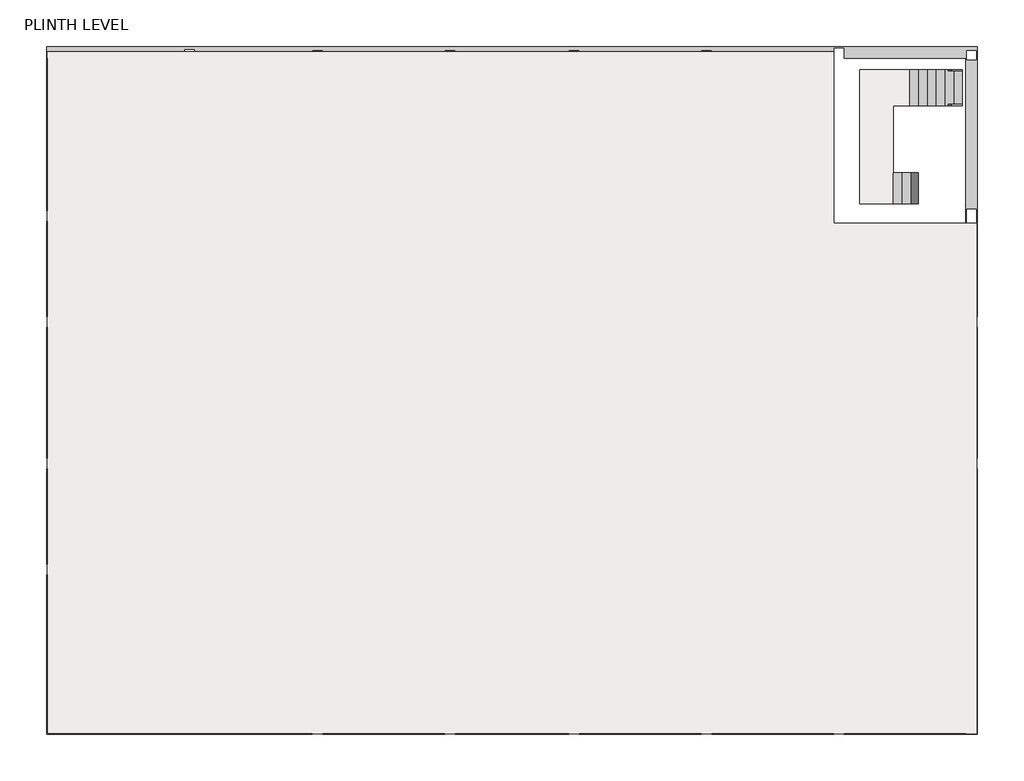
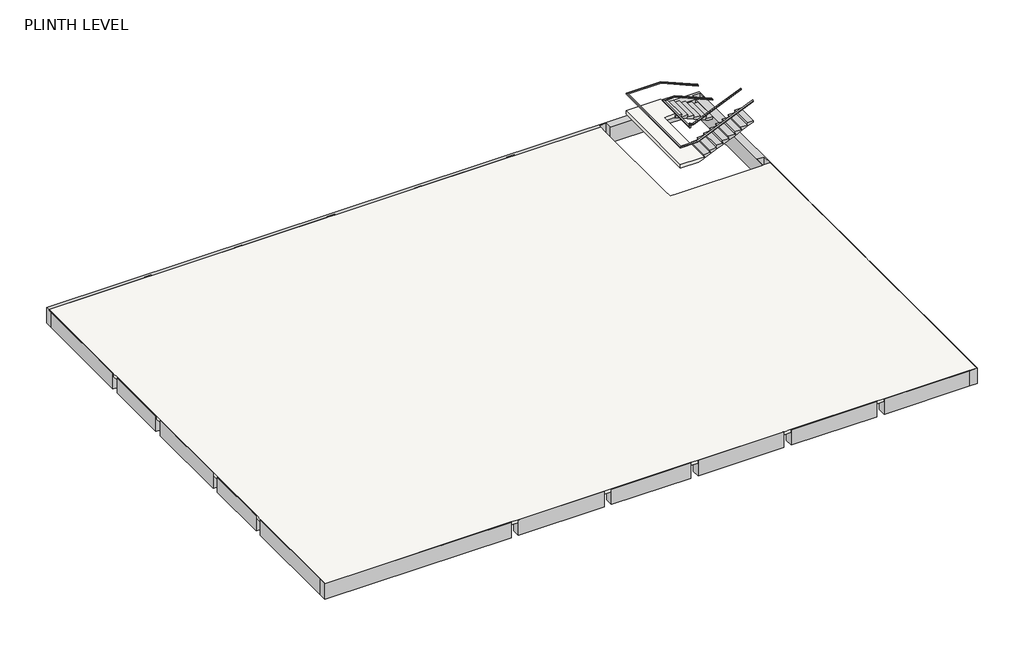
# One storey: 4 beams, 2 railings, 2 slabs, 2 stair flights.
"""IFC4 building model written with IfcOpenShell, lengths in millimetres."""

from ifc_helpers import new_model, si_unit, origin, place, context, project, spatial, faceted_brep, element, save

model = new_model("IFC4")

# Units and contexts
model_context = context("Model", 3, world=origin())
ifc_project = project(units=[si_unit("LENGTHUNIT", "METRE", prefix="MILLI")], contexts=[model_context])

# Site, building, storey
site = spatial("IfcSite", under=ifc_project)
building = spatial("IfcBuilding", under=site)
storey = spatial("IfcBuildingStorey", under=building, Name="PLINTH LEVEL", Elevation=914.4)

# Beams
placement = place(None, origin())
element("IfcBeam", 1, ObjectType="M_Concrete-Rectangular Beam : 400 x 800mm", at=placement, inside=storey, context=model_context, shape_type="Brep", body=[
    faceted_brep([(-25679.3491019, 17094.7690835, 914.4), (-20954.9491019, 17094.7690835, 914.4), (-20954.9491019, 17170.9690835, 914.4), (-20599.3491019, 17170.9690835, 914.4), (-20599.3491019, 17094.7690835, 914.4), (-16535.3491019, 17094.7690835, 914.4), (-16535.3491019, 17145.5690835, 914.4), (-16179.7491019, 17145.5690835, 914.4), (-16179.7491019, 17094.7690835, 914.4), (-11963.3491019, 17094.7690835, 914.4), (-11963.3491019, 17145.5690835, 914.4), (-11607.7491019, 17145.5690835, 914.4), (-11607.7491019, 17094.7690835, 914.4), (-7696.1491019, 17094.7690835, 914.4), (-7696.1491019, 17145.5690835, 914.4), (-7340.5491019, 17145.5690835, 914.4), (-7340.5491019, 17094.7690835, 914.4), (-3124.1491019, 17094.7690835, 914.4), (-3124.1491019, 17145.5690835, 914.4), (-2768.5491019, 17145.5690835, 914.4), (-2768.5491019, 17094.7690835, 914.4), (1447.8508981, 17094.7690835, 914.4), (1447.8508981, 17221.7690835, 914.4), (1803.4508981, 17221.7690835, 914.4), (1803.4508981, 16869.3690835, 914.4), (1825.6508981, 16869.3690835, 914.4), (5997.6508981, 16869.3690835, 914.4), (6019.8508981, 16869.3690835, 914.4), (6019.8508981, 17145.5690835, 914.4), (6375.4508981, 17145.5690835, 914.4), (6375.4508981, 16869.3690835, 914.4), (6397.6508981, 16869.3690835, 914.4), (6397.6508981, 17269.3690835, 914.4), (-25701.5491019, 17269.3690835, 914.4), (-25701.5491019, 16869.3690835, 914.4), (-25679.3491019, 16869.3690835, 914.4), (6397.6508981, 16869.3690835, 114.4), (6375.4508981, 16869.3690835, 114.4), (-25323.7491019, 16869.3690835, 114.4), (-25323.7491019, 17094.7690835, 114.4), (-25679.3491019, 17094.7690835, 114.4), (-25679.3491019, 16869.3690835, 114.4), (-25701.5491019, 16869.3690835, 114.4), (-25701.5491019, 17269.3690835, 114.4), (6397.6508981, 17269.3690835, 114.4), (6375.4508981, 17145.5690835, 114.4), (6019.8508981, 17145.5690835, 114.4), (6019.8508981, 16869.3690835, 114.4), (5997.6508981, 16869.3690835, 114.4), (1825.6508981, 16869.3690835, 114.4), (1803.4508981, 16869.3690835, 114.4), (1803.4508981, 17221.7690835, 114.4), (1447.8508981, 17221.7690835, 114.4), (1447.8508981, 16869.3690835, 114.4), (1425.6508981, 16869.3690835, 114.4), (-2746.3491019, 16869.3690835, 114.4), (-2768.5491019, 16869.3690835, 114.4), (-2768.5491019, 17145.5690835, 114.4), (-3124.1491019, 17145.5690835, 114.4), (-3124.1491019, 16869.3690835, 114.4), (-3146.3491019, 16869.3690835, 114.4), (-7318.3491019, 16869.3690835, 114.4), (-7340.5491019, 16869.3690835, 114.4), (-7340.5491019, 17145.5690835, 114.4), (-7696.1491019, 17145.5690835, 114.4), (-7696.1491019, 16869.3690835, 114.4), (-7718.3491019, 16869.3690835, 114.4), (-11585.5491019, 16869.3690835, 114.4), (-11607.7491019, 16869.3690835, 114.4), (-11607.7491019, 17145.5690835, 114.4), (-11963.3491019, 17145.5690835, 114.4), (-11963.3491019, 16869.3690835, 114.4), (-11985.5491019, 16869.3690835, 114.4), (-16157.5491019, 16869.3690835, 114.4), (-16179.7491019, 16869.3690835, 114.4), (-16179.7491019, 17145.5690835, 114.4), (-16535.3491019, 17145.5690835, 114.4), (-16535.3491019, 16869.3690835, 114.4), (-16557.5491019, 16869.3690835, 114.4), (-20577.1491019, 16869.3690835, 114.4), (-20599.3491019, 16869.3690835, 114.4), (-20599.3491019, 17170.9690835, 114.4), (-20954.9491019, 17170.9690835, 114.4), (-20954.9491019, 16869.3690835, 114.4), (-20977.1491019, 16869.3690835, 114.4), (-25301.5491019, 16869.3690835, 114.4), (-25323.7491019, 16869.3690835, 762.0), (-25323.7491019, 17094.7690835, 762.0), (-2768.5491019, 17094.7690835, 762.0), (1447.8508981, 17094.7690835, 762.0), (-16179.7491019, 16869.3690835, 762.0), (-16179.7491019, 17094.7690835, 762.0), (-16535.3491019, 17094.7690835, 762.0), (-16535.3491019, 16869.3690835, 762.0), (-11607.7491019, 16869.3690835, 762.0), (-11607.7491019, 17094.7690835, 762.0), (-11963.3491019, 17094.7690835, 762.0), (-11963.3491019, 16869.3690835, 762.0), (-7340.5491019, 16869.3690835, 762.0), (-7340.5491019, 17094.7690835, 762.0), (-7696.1491019, 17094.7690835, 762.0), (-7696.1491019, 16869.3690835, 762.0), (-2768.5491019, 16869.3690835, 762.0), (-3124.1491019, 17094.7690835, 762.0), (-3124.1491019, 16869.3690835, 762.0), (-20599.3491019, 16869.3690835, 762.0), (-20599.3491019, 17094.7690835, 762.0), (-20954.9491019, 17094.7690835, 762.0), (-20954.9491019, 16869.3690835, 762.0), (1447.8508981, 16869.3690835, 762.0), (-25679.3491019, 17094.7690835, 762.0), (-25679.3491019, 16869.3690835, 762.0), (-2746.3491019, 16869.3690835, 762.0), (1425.6508981, 16869.3690835, 762.0), (-7318.3491019, 16869.3690835, 762.0), (-3146.3491019, 16869.3690835, 762.0), (-11585.5491019, 16869.3690835, 762.0), (-7718.3491019, 16869.3690835, 762.0), (-16157.5491019, 16869.3690835, 762.0), (-11985.5491019, 16869.3690835, 762.0), (-20577.1491019, 16869.3690835, 762.0), (-16557.5491019, 16869.3690835, 762.0), (-25301.5491019, 16869.3690835, 762.0), (-20977.1491019, 16869.3690835, 762.0)], [[[0, 1, 2, 3, 4, 5, 6, 7, 8, 9, 10, 11, 12, 13, 14, 15, 16, 17, 18, 19, 20, 21, 22, 23, 24, 25, 26, 27, 28, 29, 30, 31, 32, 33, 34, 35]], [[36, 31, 30, 37]], [[38, 39, 40, 41, 42, 43, 44, 36, 37, 45, 46, 47, 48, 49, 50, 51, 52, 53, 54, 55, 56, 57, 58, 59, 60, 61, 62, 63, 64, 65, 66, 67, 68, 69, 70, 71, 72, 73, 74, 75, 76, 77, 78, 79, 80, 81, 82, 83, 84, 85]], [[43, 33, 32, 44]], [[39, 38, 86, 87]], [[88, 89, 21, 20]], [[28, 27, 47, 46]], [[75, 74, 90, 91, 8, 7]], [[77, 76, 6, 5, 92, 93]], [[69, 68, 94, 95, 12, 11]], [[71, 70, 10, 9, 96, 97]], [[63, 62, 98, 99, 16, 15]], [[65, 64, 14, 13, 100, 101]], [[57, 56, 102, 88, 20, 19]], [[59, 58, 18, 17, 103, 104]], [[3, 81, 80, 105, 106, 4]], [[82, 2, 1, 107, 108, 83]], [[24, 23, 51, 50]], [[53, 52, 22, 21, 89, 109]], [[30, 29, 45, 37]], [[34, 33, 43, 42]], [[40, 110, 0, 35, 111, 41]], [[32, 31, 36, 44]], [[89, 88, 102, 112, 113, 109]], [[99, 103, 17, 16]], [[95, 100, 13, 12]], [[91, 96, 9, 8]], [[106, 92, 5, 4]], [[40, 39, 87, 107, 1, 0, 110]], [[103, 99, 98, 114, 115, 104]], [[100, 95, 94, 116, 117, 101]], [[96, 91, 90, 118, 119, 97]], [[92, 106, 105, 120, 121, 93]], [[107, 87, 86, 122, 123, 108]], [[34, 42, 41, 111, 35]], [[28, 46, 45, 29]], [[47, 27, 26, 25, 24, 50, 49, 48]], [[6, 76, 75, 7]], [[80, 79, 78, 77, 93, 121, 120, 105]], [[10, 70, 69, 11]], [[74, 73, 72, 71, 97, 119, 118, 90]], [[14, 64, 63, 15]], [[68, 67, 66, 65, 101, 117, 116, 94]], [[18, 58, 57, 19]], [[62, 61, 60, 59, 104, 115, 114, 98]], [[2, 82, 81, 3]], [[38, 85, 84, 83, 108, 123, 122, 86]], [[22, 52, 51, 23]], [[56, 55, 54, 53, 109, 113, 112, 102]]]),
])
element("IfcBeam", 2, ObjectType="M_Concrete-Rectangular Beam : 400 x 800mm", at=placement, inside=storey, context=model_context, shape_type="Brep", body=[
    faceted_brep([(5997.6508981, -6447.8309165, 914.4), (6397.6508981, -6447.8309165, 914.4), (6397.6508981, 2718.3690835, 914.4), (6375.4508981, 2718.3690835, 914.4), (6375.4508981, -6425.6309165, 914.4), (5997.6508981, -6425.6309165, 914.4), (5997.6508981, -6447.8309165, 114.4), (5997.6508981, -6425.6309165, 762.0), (5997.6508981, -6047.8309165, 762.0), (5997.6508981, -961.4309165, 762.0), (5997.6508981, -561.4309165, 762.0), (5997.6508981, 2696.1690835, 762.0), (5997.6508981, 2718.3690835, 762.0), (5997.6508981, 2718.3690835, 114.4), (5997.6508981, 2696.1690835, 114.4), (5997.6508981, -561.4309165, 114.4), (5997.6508981, -961.4309165, 114.4), (5997.6508981, -6047.8309165, 114.4), (6397.6508981, 2718.3690835, 114.4), (6397.6508981, -6447.8309165, 114.4), (6375.4508981, -6425.6309165, 114.4), (6375.4508981, -6070.0309165, 114.4), (6019.8508981, -6070.0309165, 114.4), (6019.8508981, -6425.6309165, 114.4), (6375.4508981, -1015.4309165, 114.4), (6375.4508981, -507.4309165, 114.4), (6019.8508981, -507.4309165, 114.4), (6019.8508981, -1015.4309165, 114.4), (6375.4508981, -6425.6309165, 762.0), (6375.4508981, 2718.3690835, 762.0), (6375.4508981, -507.4309165, 762.0), (6375.4508981, -1015.4309165, 762.0), (6375.4508981, -6070.0309165, 762.0), (6019.8508981, -6070.0309165, 762.0), (6019.8508981, -6425.6309165, 762.0), (6019.8508981, -1015.4309165, 762.0), (6019.8508981, -507.4309165, 762.0)], [[[0, 1, 2, 3, 4, 5]], [[6, 0, 5, 7, 8, 9, 10, 11, 12, 13, 14, 15, 16, 17]], [[13, 18, 19, 6, 17, 16, 15, 14], [20, 21, 22, 23], [24, 25, 26, 27]], [[18, 2, 1, 19]], [[21, 20, 28, 4, 3, 29, 30, 25, 24, 31, 32]], [[23, 22, 33, 34]], [[22, 21, 32, 33]], [[18, 13, 12, 29, 3, 2]], [[24, 27, 35, 31]], [[27, 26, 36, 35]], [[26, 25, 30, 36]], [[1, 0, 6, 19]], [[20, 23, 34, 7, 5, 4, 28]], [[7, 34, 33, 32, 31, 35, 36, 30, 29, 12, 11, 10, 9, 8]]]),
    faceted_brep([(6397.6508981, 16869.3690835, 914.4), (6397.6508981, 16869.3690835, 114.4), (6375.4508981, 16869.3690835, 114.4), (6375.4508981, 16869.3690835, 914.4), (5997.6508981, 7950.7690835, 114.4), (6397.6508981, 7950.7690835, 114.4), (6397.6508981, 7950.7690835, 914.4), (6375.4508981, 7950.7690835, 914.4), (6375.4508981, 7950.7690835, 762.0), (5997.6508981, 7950.7690835, 762.0), (6019.8508981, 11176.5690835, 914.4), (6019.8508981, 11684.5690835, 914.4), (6375.4508981, 11684.5690835, 914.4), (6375.4508981, 11176.5690835, 914.4), (6375.4508981, 16789.9690835, 914.4), (6019.8508981, 16789.9690835, 914.4), (6019.8508981, 16869.3690835, 914.4), (5997.6508981, 16869.3690835, 914.4), (5997.6508981, 11630.5690835, 914.4), (5997.6508981, 11230.5690835, 914.4), (5997.6508981, 11176.5690835, 914.4), (5997.6508981, 16869.3690835, 114.4), (5997.6508981, 11630.5690835, 114.4), (5997.6508981, 11230.5690835, 114.4), (5997.6508981, 7972.9690835, 114.4), (5997.6508981, 7972.9690835, 762.0), (5997.6508981, 11176.5690835, 762.0), (6019.8508981, 16869.3690835, 114.4), (6019.8508981, 16789.9690835, 114.4), (6375.4508981, 16789.9690835, 114.4), (6375.4508981, 11176.5690835, 114.4), (6375.4508981, 11684.5690835, 114.4), (6019.8508981, 11684.5690835, 114.4), (6019.8508981, 11176.5690835, 114.4), (6019.8508981, 11176.5690835, 762.0), (6375.4508981, 11176.5690835, 762.0)], [[[0, 1, 2, 3]], [[4, 5, 6, 7, 8, 9]], [[10, 11, 12, 13, 7, 6, 0, 3, 14, 15, 16, 17, 18, 19, 20]], [[17, 21, 22, 23, 24, 4, 9, 25, 26, 20, 19, 18]], [[5, 4, 24, 23, 22, 21, 27, 28, 29, 2, 1], [30, 31, 32, 33]], [[6, 5, 1, 0]], [[30, 33, 34, 35]], [[32, 11, 10, 34, 33]], [[11, 32, 31, 12]], [[9, 8, 35, 34, 26, 25]], [[12, 31, 30, 35, 8, 7, 13]], [[29, 14, 3, 2]], [[14, 29, 28, 15]], [[15, 28, 27, 16]], [[21, 17, 16, 27]], [[26, 34, 10, 20]]]),
    faceted_brep([(6397.6508981, 7595.1690835, 114.4), (5997.6508981, 7595.1690835, 114.4), (5997.6508981, 7595.1690835, 762.0), (6375.4508981, 7595.1690835, 762.0), (6375.4508981, 7595.1690835, 914.4), (6397.6508981, 7595.1690835, 914.4), (5997.6508981, 3073.9690835, 114.4), (6397.6508981, 3073.9690835, 114.4), (6397.6508981, 3073.9690835, 914.4), (6375.4508981, 3073.9690835, 914.4), (6375.4508981, 3073.9690835, 762.0), (5997.6508981, 3073.9690835, 762.0), (5997.6508981, 7572.9690835, 114.4), (5997.6508981, 3096.1690835, 114.4), (5997.6508981, 3096.1690835, 762.0), (5997.6508981, 7572.9690835, 762.0)], [[[0, 1, 2, 3, 4, 5]], [[6, 7, 8, 9, 10, 11]], [[8, 5, 4, 9]], [[1, 12, 13, 6, 11, 14, 15, 2]], [[1, 0, 7, 6, 13, 12]], [[0, 5, 8, 7]], [[4, 3, 10, 9]], [[3, 2, 15, 14, 11, 10]]]),
])
element("IfcBeam", 3, ObjectType="M_Concrete-Rectangular Beam : 400 x 800mm", at=placement, inside=storey, context=model_context, shape_type="Brep", body=[
    faceted_brep([(-16535.3491019, -6425.6309165, 914.4), (-25679.3491019, -6425.6309165, 914.4), (-25679.3491019, -6047.8309165, 914.4), (-25701.5491019, -6047.8309165, 914.4), (-25701.5491019, -6447.8309165, 914.4), (-16535.3491019, -6447.8309165, 914.4), (-25701.5491019, -6047.8309165, 114.4), (-25679.3491019, -6047.8309165, 762.0), (-25301.5491019, -6047.8309165, 762.0), (-20977.1491019, -6047.8309165, 762.0), (-20577.1491019, -6047.8309165, 762.0), (-16557.5491019, -6047.8309165, 762.0), (-16535.3491019, -6047.8309165, 762.0), (-16535.3491019, -6047.8309165, 114.4), (-16557.5491019, -6047.8309165, 114.4), (-20577.1491019, -6047.8309165, 114.4), (-20977.1491019, -6047.8309165, 114.4), (-25301.5491019, -6047.8309165, 114.4), (-16535.3491019, -6447.8309165, 114.4), (-25701.5491019, -6447.8309165, 114.4), (-25323.7491019, -6425.6309165, 114.4), (-25323.7491019, -6070.0309165, 114.4), (-25679.3491019, -6070.0309165, 114.4), (-25679.3491019, -6425.6309165, 114.4), (-20599.3491019, -6425.6309165, 114.4), (-20599.3491019, -6070.0309165, 114.4), (-20954.9491019, -6070.0309165, 114.4), (-20954.9491019, -6425.6309165, 114.4), (-25323.7491019, -6425.6309165, 762.0), (-25323.7491019, -6070.0309165, 762.0), (-16535.3491019, -6425.6309165, 762.0), (-20599.3491019, -6425.6309165, 762.0), (-20954.9491019, -6425.6309165, 762.0), (-25679.3491019, -6425.6309165, 762.0), (-25679.3491019, -6070.0309165, 762.0), (-20599.3491019, -6070.0309165, 762.0), (-20954.9491019, -6070.0309165, 762.0)], [[[0, 1, 2, 3, 4, 5]], [[6, 3, 2, 7, 8, 9, 10, 11, 12, 13, 14, 15, 16, 17]], [[13, 18, 19, 6, 17, 16, 15, 14], [20, 21, 22, 23], [24, 25, 26, 27]], [[18, 5, 4, 19]], [[21, 20, 28, 29]], [[30, 31, 24, 27, 32, 28, 20, 23, 33, 1, 0]], [[22, 21, 29, 34]], [[25, 24, 31, 35]], [[27, 26, 36, 32]], [[26, 25, 35, 36]], [[18, 13, 12, 30, 0, 5]], [[4, 3, 6, 19]], [[1, 33, 23, 22, 34, 7, 2]], [[28, 32, 36, 35, 31, 30, 12, 11, 10, 9, 8, 7, 34, 29]]]),
    faceted_brep([(5997.6508981, -6447.8309165, 114.4), (5997.6508981, -6047.8309165, 114.4), (5997.6508981, -6047.8309165, 762.0), (5997.6508981, -6425.6309165, 762.0), (5997.6508981, -6425.6309165, 914.4), (5997.6508981, -6447.8309165, 914.4), (1803.4508981, -6047.8309165, 114.4), (1803.4508981, -6447.8309165, 114.4), (1803.4508981, -6447.8309165, 914.4), (1803.4508981, -6425.6309165, 914.4), (1803.4508981, -6425.6309165, 762.0), (1803.4508981, -6047.8309165, 762.0), (1825.6508981, -6047.8309165, 114.4), (1825.6508981, -6047.8309165, 762.0)], [[[0, 1, 2, 3, 4, 5]], [[6, 7, 8, 9, 10, 11]], [[8, 5, 4, 9]], [[1, 12, 6, 11, 13, 2]], [[1, 0, 7, 6, 12]], [[0, 5, 8, 7]], [[10, 3, 2, 13, 11]], [[3, 10, 9, 4]]]),
    faceted_brep([(-16179.7491019, -6047.8309165, 114.4), (-16179.7491019, -6447.8309165, 114.4), (-16179.7491019, -6447.8309165, 914.4), (-16179.7491019, -6425.6309165, 914.4), (-16179.7491019, -6425.6309165, 762.0), (-16179.7491019, -6047.8309165, 762.0), (-11963.3491019, -6447.8309165, 914.4), (-11963.3491019, -6425.6309165, 914.4), (-11963.3491019, -6047.8309165, 114.4), (-11985.5491019, -6047.8309165, 114.4), (-16157.5491019, -6047.8309165, 114.4), (-16157.5491019, -6047.8309165, 762.0), (-11985.5491019, -6047.8309165, 762.0), (-11963.3491019, -6047.8309165, 762.0), (-11963.3491019, -6447.8309165, 114.4), (-11963.3491019, -6425.6309165, 762.0)], [[[0, 1, 2, 3, 4, 5]], [[2, 6, 7, 3]], [[8, 9, 10, 0, 5, 11, 12, 13]], [[1, 0, 10, 9, 8, 14]], [[2, 1, 14, 6]], [[14, 8, 13, 15, 7, 6]], [[15, 4, 3, 7]], [[4, 15, 13, 12, 11, 5]]]),
    faceted_brep([(-11607.7491019, -6047.8309165, 114.4), (-11607.7491019, -6447.8309165, 114.4), (-11607.7491019, -6447.8309165, 914.4), (-11607.7491019, -6425.6309165, 914.4), (-11607.7491019, -6425.6309165, 762.0), (-11607.7491019, -6047.8309165, 762.0), (-7696.1491019, -6447.8309165, 914.4), (-7696.1491019, -6425.6309165, 914.4), (-7696.1491019, -6047.8309165, 114.4), (-7718.3491019, -6047.8309165, 114.4), (-11585.5491019, -6047.8309165, 114.4), (-11585.5491019, -6047.8309165, 762.0), (-7718.3491019, -6047.8309165, 762.0), (-7696.1491019, -6047.8309165, 762.0), (-7696.1491019, -6447.8309165, 114.4), (-7696.1491019, -6425.6309165, 762.0)], [[[0, 1, 2, 3, 4, 5]], [[2, 6, 7, 3]], [[8, 9, 10, 0, 5, 11, 12, 13]], [[1, 0, 10, 9, 8, 14]], [[2, 1, 14, 6]], [[14, 8, 13, 15, 7, 6]], [[15, 4, 3, 7]], [[4, 15, 13, 12, 11, 5]]]),
    faceted_brep([(-7340.5491019, -6047.8309165, 114.4), (-7340.5491019, -6447.8309165, 114.4), (-7340.5491019, -6447.8309165, 914.4), (-7340.5491019, -6425.6309165, 914.4), (-7340.5491019, -6425.6309165, 762.0), (-7340.5491019, -6047.8309165, 762.0), (-3124.1491019, -6447.8309165, 914.4), (-3124.1491019, -6425.6309165, 914.4), (-3124.1491019, -6047.8309165, 114.4), (-3146.3491019, -6047.8309165, 114.4), (-7318.3491019, -6047.8309165, 114.4), (-7318.3491019, -6047.8309165, 762.0), (-3146.3491019, -6047.8309165, 762.0), (-3124.1491019, -6047.8309165, 762.0), (-3124.1491019, -6447.8309165, 114.4), (-3124.1491019, -6425.6309165, 762.0)], [[[0, 1, 2, 3, 4, 5]], [[2, 6, 7, 3]], [[8, 9, 10, 0, 5, 11, 12, 13]], [[1, 0, 10, 9, 8, 14]], [[2, 1, 14, 6]], [[14, 8, 13, 15, 7, 6]], [[15, 4, 3, 7]], [[4, 15, 13, 12, 11, 5]]]),
    faceted_brep([(-2768.5491019, -6047.8309165, 114.4), (-2768.5491019, -6447.8309165, 114.4), (-2768.5491019, -6447.8309165, 914.4), (-2768.5491019, -6425.6309165, 914.4), (-2768.5491019, -6425.6309165, 762.0), (-2768.5491019, -6047.8309165, 762.0), (1447.8508981, -6447.8309165, 914.4), (1447.8508981, -6425.6309165, 914.4), (1447.8508981, -6047.8309165, 114.4), (1425.6508981, -6047.8309165, 114.4), (-2746.3491019, -6047.8309165, 114.4), (-2746.3491019, -6047.8309165, 762.0), (1425.6508981, -6047.8309165, 762.0), (1447.8508981, -6047.8309165, 762.0), (1447.8508981, -6447.8309165, 114.4), (1447.8508981, -6425.6309165, 762.0)], [[[0, 1, 2, 3, 4, 5]], [[2, 6, 7, 3]], [[8, 9, 10, 0, 5, 11, 12, 13]], [[1, 0, 10, 9, 8, 14]], [[2, 1, 14, 6]], [[14, 8, 13, 15, 7, 6]], [[15, 4, 3, 7]], [[4, 15, 13, 12, 11, 5]]]),
])
element("IfcBeam", 4, ObjectType="M_Concrete-Rectangular Beam : 400 x 800mm", at=placement, inside=storey, context=model_context, shape_type="Brep", body=[
    faceted_brep([(-25701.5491019, -939.2309165, 914.4), (-25701.5491019, -6047.8309165, 914.4), (-25679.3491019, -6047.8309165, 914.4), (-25679.3491019, -939.2309165, 914.4), (-25301.5491019, -6047.8309165, 114.4), (-25301.5491019, -961.4309165, 114.4), (-25301.5491019, -939.2309165, 114.4), (-25301.5491019, -939.2309165, 762.0), (-25301.5491019, -961.4309165, 762.0), (-25301.5491019, -6047.8309165, 762.0), (-25701.5491019, -6047.8309165, 114.4), (-25701.5491019, -939.2309165, 114.4), (-25679.3491019, -6047.8309165, 762.0), (-25679.3491019, -939.2309165, 762.0)], [[[0, 1, 2, 3]], [[4, 5, 6, 7, 8, 9]], [[4, 10, 11, 6, 5]], [[10, 1, 0, 11]], [[10, 4, 9, 12, 2, 1]], [[13, 7, 6, 11, 0, 3]], [[12, 13, 3, 2]], [[13, 12, 9, 8, 7]]]),
    faceted_brep([(-25301.5491019, 16869.3690835, 762.0), (-25301.5491019, 16869.3690835, 114.4), (-25323.7491019, 16869.3690835, 114.4), (-25323.7491019, 16869.3690835, 762.0), (-25701.5491019, 16869.3690835, 914.4), (-25701.5491019, 11608.3690835, 914.4), (-25679.3491019, 11608.3690835, 914.4), (-25679.3491019, 16869.3690835, 914.4), (-25301.5491019, 11608.3690835, 114.4), (-25301.5491019, 11630.5690835, 114.4), (-25301.5491019, 11630.5690835, 762.0), (-25301.5491019, 11608.3690835, 762.0), (-25701.5491019, 11608.3690835, 114.4), (-25701.5491019, 16869.3690835, 114.4), (-25679.3491019, 16869.3690835, 114.4), (-25679.3491019, 16739.1690835, 114.4), (-25323.7491019, 16739.1690835, 114.4), (-25679.3491019, 11608.3690835, 762.0), (-25323.7491019, 16739.1690835, 762.0), (-25679.3491019, 16739.1690835, 762.0)], [[[0, 1, 2, 3]], [[4, 5, 6, 7]], [[8, 9, 1, 0, 10, 11]], [[1, 9, 8, 12, 13, 14, 15, 16, 2]], [[4, 13, 12, 5]], [[11, 17, 6, 5, 12, 8]], [[11, 10, 0, 3, 18, 19, 17]], [[6, 17, 19, 15, 14, 7]], [[16, 18, 3, 2]], [[18, 16, 15, 19]], [[13, 4, 7, 14]]]),
    faceted_brep([(-25701.5491019, 7950.7690835, 114.4), (-25301.5491019, 7950.7690835, 114.4), (-25301.5491019, 7950.7690835, 762.0), (-25679.3491019, 7950.7690835, 762.0), (-25679.3491019, 7950.7690835, 914.4), (-25701.5491019, 7950.7690835, 914.4), (-25679.3491019, 11252.7690835, 762.0), (-25301.5491019, 11252.7690835, 762.0), (-25301.5491019, 11252.7690835, 114.4), (-25701.5491019, 11252.7690835, 114.4), (-25701.5491019, 11252.7690835, 914.4), (-25679.3491019, 11252.7690835, 914.4), (-25301.5491019, 7972.9690835, 762.0), (-25301.5491019, 11230.5690835, 762.0), (-25301.5491019, 7972.9690835, 114.4), (-25301.5491019, 11230.5690835, 114.4)], [[[0, 1, 2, 3, 4, 5]], [[6, 7, 8, 9, 10, 11]], [[6, 3, 2, 12, 13, 7]], [[3, 6, 11, 4]], [[10, 5, 4, 11]], [[1, 14, 15, 8, 7, 13, 12, 2]], [[1, 0, 9, 8, 15, 14]], [[0, 5, 10, 9]]]),
    faceted_brep([(-25301.5491019, 7595.1690835, 114.4), (-25701.5491019, 7595.1690835, 114.4), (-25701.5491019, 7595.1690835, 914.4), (-25679.3491019, 7595.1690835, 914.4), (-25679.3491019, 7595.1690835, 762.0), (-25301.5491019, 7595.1690835, 762.0), (-25301.5491019, 3073.9690835, 762.0), (-25679.3491019, 3073.9690835, 762.0), (-25679.3491019, 3073.9690835, 914.4), (-25701.5491019, 3073.9690835, 914.4), (-25701.5491019, 3073.9690835, 114.4), (-25301.5491019, 3073.9690835, 114.4), (-25301.5491019, 3096.1690835, 762.0), (-25301.5491019, 7572.9690835, 762.0), (-25301.5491019, 3096.1690835, 114.4), (-25301.5491019, 7572.9690835, 114.4)], [[[0, 1, 2, 3, 4, 5]], [[6, 7, 8, 9, 10, 11]], [[4, 7, 6, 12, 13, 5]], [[7, 4, 3, 8]], [[2, 9, 8, 3]], [[11, 14, 15, 0, 5, 13, 12, 6]], [[1, 0, 15, 14, 11, 10]], [[2, 1, 10, 9]]]),
    faceted_brep([(-25679.3491019, 2718.3690835, 762.0), (-25301.5491019, 2718.3690835, 762.0), (-25301.5491019, 2718.3690835, 114.4), (-25701.5491019, 2718.3690835, 114.4), (-25701.5491019, 2718.3690835, 914.4), (-25679.3491019, 2718.3690835, 914.4), (-25301.5491019, -583.6309165, 762.0), (-25679.3491019, -583.6309165, 762.0), (-25679.3491019, -583.6309165, 914.4), (-25701.5491019, -583.6309165, 914.4), (-25701.5491019, -583.6309165, 114.4), (-25301.5491019, -583.6309165, 114.4), (-25301.5491019, -561.4309165, 762.0), (-25301.5491019, 2696.1690835, 762.0), (-25301.5491019, -561.4309165, 114.4), (-25301.5491019, 2696.1690835, 114.4)], [[[0, 1, 2, 3, 4, 5]], [[6, 7, 8, 9, 10, 11]], [[0, 7, 6, 12, 13, 1]], [[7, 0, 5, 8]], [[4, 9, 8, 5]], [[11, 14, 15, 2, 1, 13, 12, 6]], [[2, 15, 14, 11, 10, 3]], [[9, 4, 3, 10]]]),
])

# Railings
element("IfcRailing", 5, ObjectType="Handrail", at=placement, inside=storey, context=model_context, shape_type="Brep", body=[
    faceted_brep([(5878.2258195, 16426.305974, 1958.975), (5878.2258195, 16426.305974, 1903.7359813), (5878.2258195, 16477.105974, 1903.7359813), (5878.2258195, 16477.105974, 1958.975), (4049.4258195, 16426.305974, 2740.025), (4039.0320197, 16426.305974, 2689.225), (4039.0320197, 16477.105974, 2689.225), (4049.4258195, 16477.105974, 2740.025), (2398.4258195, 16426.305974, 2740.025), (2398.4258195, 16426.305974, 2689.225), (2347.6258195, 16477.105974, 2689.225), (2347.6258195, 16477.105974, 2740.025), (2398.4258195, 11896.1816424, 2740.025), (2398.4258195, 11896.1816424, 2689.225), (2347.6258195, 11845.3816424, 2689.225), (2347.6258195, 11845.3816424, 2740.025), (3188.2923097, 11896.1816424, 2740.025), (3198.6861096, 11896.1816424, 2689.225), (3198.6861096, 11845.3816424, 2689.225), (3188.2923097, 11845.3816424, 2740.025), (5931.4923097, 11896.1816424, 3911.6), (5931.4923097, 11845.3816424, 3911.6), (5931.4923097, 11845.3816424, 3856.3609813), (5931.4923097, 11896.1816424, 3856.3609813)], [[[0, 1, 2, 3]], [[1, 0, 4, 5]], [[2, 1, 5, 6]], [[3, 2, 6, 7]], [[0, 3, 7, 4]], [[5, 4, 8, 9]], [[6, 5, 9, 10]], [[7, 6, 10, 11]], [[4, 7, 11, 8]], [[9, 8, 12, 13]], [[10, 9, 13, 14]], [[11, 10, 14, 15]], [[8, 11, 15, 12]], [[13, 12, 16, 17]], [[14, 13, 17, 18]], [[15, 14, 18, 19]], [[12, 15, 19, 16]], [[20, 21, 22, 23]], [[17, 16, 20, 23]], [[18, 17, 23, 22]], [[19, 18, 22, 21]], [[16, 19, 21, 20]]]),
])
element("IfcRailing", 6, ObjectType="Handrail", at=placement, inside=storey, context=model_context, shape_type="Brep", body=[
    faceted_brep([(5878.2258195, 15223.6852874, 1958.975), (5878.2258195, 15223.6852874, 1903.7359813), (5878.2258195, 15274.4852874, 1903.7359813), (5878.2258195, 15274.4852874, 1958.975), (4049.4258195, 15223.6852874, 2740.025), (4039.0320197, 15223.6852874, 2689.225), (4039.0320197, 15274.4852874, 2689.225), (4049.4258195, 15274.4852874, 2740.025), (3493.0923097, 15223.6852874, 2740.025), (3493.0923097, 15223.6852874, 2689.225), (3442.2923097, 15274.4852874, 2689.225), (3442.2923097, 15274.4852874, 2740.025), (3493.0923097, 12985.9409784, 2740.025), (3493.0923097, 12935.1409784, 2689.225), (3442.2923097, 12935.1409784, 2689.225), (3442.2923097, 12985.9409784, 2740.025), (3493.0923097, 12985.9409784, 2902.74375), (3493.0923097, 12935.1409784, 2851.94375), (3442.2923097, 12935.1409784, 2851.94375), (3442.2923097, 12985.9409784, 2902.74375), (3493.0923097, 12909.7409784, 2902.74375), (3493.0923097, 12909.7409784, 2851.94375), (3442.2923097, 12858.9409784, 2851.94375), (3442.2923097, 12858.9409784, 2902.74375), (3569.2923097, 12909.7409784, 2902.74375), (3579.6861096, 12909.7409784, 2851.94375), (3579.6861096, 12858.9409784, 2851.94375), (3569.2923097, 12858.9409784, 2902.74375), (5931.4923097, 12909.7409784, 3911.6), (5931.4923097, 12858.9409784, 3911.6), (5931.4923097, 12858.9409784, 3856.3609813), (5931.4923097, 12909.7409784, 3856.3609813)], [[[0, 1, 2, 3]], [[1, 0, 4, 5]], [[2, 1, 5, 6]], [[3, 2, 6, 7]], [[0, 3, 7, 4]], [[5, 4, 8, 9]], [[6, 5, 9, 10]], [[7, 6, 10, 11]], [[4, 7, 11, 8]], [[9, 8, 12, 13]], [[10, 9, 13, 14]], [[11, 10, 14, 15]], [[8, 11, 15, 12]], [[13, 12, 16, 17]], [[14, 13, 17, 18]], [[15, 14, 18, 19]], [[12, 15, 19, 16]], [[17, 16, 20, 21]], [[18, 17, 21, 22]], [[19, 18, 22, 23]], [[16, 19, 23, 20]], [[21, 20, 24, 25]], [[22, 21, 25, 26]], [[23, 22, 26, 27]], [[20, 23, 27, 24]], [[28, 29, 30, 31]], [[25, 24, 28, 31]], [[26, 25, 31, 30]], [[27, 26, 30, 29]], [[24, 27, 29, 28]]]),
])

# Slabs
element("IfcSlab", 7, ObjectType="6\" Foundation Slab", at=placement, inside=storey, context=model_context, shape_type="Brep", body=[
    faceted_brep([(6375.4508981, -6425.6309165, 762.0), (6019.8508981, -6425.6309165, 762.0), (5997.6508981, -6425.6309165, 762.0), (1803.4508981, -6425.6309165, 762.0), (1447.8508981, -6425.6309165, 762.0), (-2768.5491019, -6425.6309165, 762.0), (-3124.1491019, -6425.6309165, 762.0), (-7340.5491019, -6425.6309165, 762.0), (-7696.1491019, -6425.6309165, 762.0), (-11607.7491019, -6425.6309165, 762.0), (-11963.3491019, -6425.6309165, 762.0), (-16179.7491019, -6425.6309165, 762.0), (-16535.3491019, -6425.6309165, 762.0), (-20599.3491019, -6425.6309165, 762.0), (-20954.9491019, -6425.6309165, 762.0), (-25323.7491019, -6425.6309165, 762.0), (-25679.3491019, -6425.6309165, 762.0), (-25679.3491019, -6070.0309165, 762.0), (-25679.3491019, -6047.8309165, 762.0), (-25679.3491019, -939.2309165, 762.0), (-25679.3491019, -583.6309165, 762.0), (-25679.3491019, 2718.3690835, 762.0), (-25679.3491019, 3073.9690835, 762.0), (-25679.3491019, 7595.1690835, 762.0), (-25679.3491019, 7950.7690835, 762.0), (-25679.3491019, 11252.7690835, 762.0), (-25679.3491019, 11608.3690835, 762.0), (-25679.3491019, 16739.1690835, 762.0), (-25679.3491019, 17094.7690835, 762.0), (-25323.7491019, 17094.7690835, 762.0), (-20954.9491019, 17094.7690835, 762.0), (-20599.3491019, 17094.7690835, 762.0), (-16535.3491019, 17094.7690835, 762.0), (-16179.7491019, 17094.7690835, 762.0), (-11963.3491019, 17094.7690835, 762.0), (-11607.7491019, 17094.7690835, 762.0), (-7696.1491019, 17094.7690835, 762.0), (-7340.5491019, 17094.7690835, 762.0), (-3124.1491019, 17094.7690835, 762.0), (-2768.5491019, 17094.7690835, 762.0), (1447.8508981, 17094.7690835, 762.0), (1447.8508981, 16869.3690835, 762.0), (1447.8508981, 16713.7690835, 762.0), (1447.8508981, 11659.1690835, 762.0), (1447.8508981, 11201.9690835, 762.0), (1447.8508981, 11176.5690835, 762.0), (1825.6508981, 11176.5690835, 762.0), (5997.6508981, 11176.5690835, 762.0), (6019.8508981, 11176.5690835, 762.0), (6375.4508981, 11176.5690835, 762.0), (6375.4508981, 7950.7690835, 762.0), (6375.4508981, 7595.1690835, 762.0), (6375.4508981, 3073.9690835, 762.0), (6375.4508981, 2718.3690835, 762.0), (6375.4508981, -507.4309165, 762.0), (6375.4508981, -1015.4309165, 762.0), (6375.4508981, -6070.0309165, 762.0), (-25679.3491019, -6425.6309165, 914.4), (-16535.3491019, -6425.6309165, 914.4), (-16179.7491019, -6425.6309165, 914.4), (-11963.3491019, -6425.6309165, 914.4), (-11607.7491019, -6425.6309165, 914.4), (-7696.1491019, -6425.6309165, 914.4), (-7340.5491019, -6425.6309165, 914.4), (-3124.1491019, -6425.6309165, 914.4), (-2768.5491019, -6425.6309165, 914.4), (1447.8508981, -6425.6309165, 914.4), (1803.4508981, -6425.6309165, 914.4), (5997.6508981, -6425.6309165, 914.4), (6375.4508981, -6425.6309165, 914.4), (6375.4508981, 2718.3690835, 914.4), (6375.4508981, 3073.9690835, 914.4), (6375.4508981, 7595.1690835, 914.4), (6375.4508981, 7950.7690835, 914.4), (6375.4508981, 11176.5690835, 914.4), (6019.8508981, 11176.5690835, 914.4), (5997.6508981, 11176.5690835, 914.4), (1825.6508981, 11176.5690835, 914.4), (1447.8508981, 11176.5690835, 914.4), (1447.8508981, 11201.9690835, 914.4), (1447.8508981, 11659.1690835, 914.4), (1447.8508981, 16713.7690835, 914.4), (1447.8508981, 17094.7690835, 914.4), (-2768.5491019, 17094.7690835, 914.4), (-3124.1491019, 17094.7690835, 914.4), (-7340.5491019, 17094.7690835, 914.4), (-7696.1491019, 17094.7690835, 914.4), (-11607.7491019, 17094.7690835, 914.4), (-11963.3491019, 17094.7690835, 914.4), (-16179.7491019, 17094.7690835, 914.4), (-16535.3491019, 17094.7690835, 914.4), (-20599.3491019, 17094.7690835, 914.4), (-20954.9491019, 17094.7690835, 914.4), (-25679.3491019, 17094.7690835, 914.4), (-25679.3491019, 16869.3690835, 914.4), (-25679.3491019, 11608.3690835, 914.4), (-25679.3491019, 11252.7690835, 914.4), (-25679.3491019, 7950.7690835, 914.4), (-25679.3491019, 7595.1690835, 914.4), (-25679.3491019, 3073.9690835, 914.4), (-25679.3491019, 2718.3690835, 914.4), (-25679.3491019, -583.6309165, 914.4), (-25679.3491019, -939.2309165, 914.4), (-25679.3491019, -6047.8309165, 914.4)], [[[0, 1, 2, 3, 4, 5, 6, 7, 8, 9, 10, 11, 12, 13, 14, 15, 16, 17, 18, 19, 20, 21, 22, 23, 24, 25, 26, 27, 28, 29, 30, 31, 32, 33, 34, 35, 36, 37, 38, 39, 40, 41, 42, 43, 44, 45, 46, 47, 48, 49, 50, 51, 52, 53, 54, 55, 56]], [[57, 58, 59, 60, 61, 62, 63, 64, 65, 66, 67, 68, 69, 70, 71, 72, 73, 74, 75, 76, 77, 78, 79, 80, 81, 82, 83, 84, 85, 86, 87, 88, 89, 90, 91, 92, 93, 94, 95, 96, 97, 98, 99, 100, 101, 102, 103]], [[69, 0, 56, 55, 54, 53, 52, 51, 50, 49, 74, 73, 72, 71, 70]], [[16, 15, 14, 13, 12, 11, 10, 9, 8, 7, 6, 5, 4, 3, 2, 1, 0, 69, 68, 67, 66, 65, 64, 63, 62, 61, 60, 59, 58, 57]], [[28, 27, 26, 25, 24, 23, 22, 21, 20, 19, 18, 17, 16, 57, 103, 102, 101, 100, 99, 98, 97, 96, 95, 94, 93]], [[28, 93, 92, 91, 90, 89, 88, 87, 86, 85, 84, 83, 82, 40, 39, 38, 37, 36, 35, 34, 33, 32, 31, 30, 29]], [[78, 45, 44, 43, 42, 41, 40, 82, 81, 80, 79]], [[45, 78, 77, 76, 75, 74, 49, 48, 47, 46]]]),
])
element("IfcSlab", 8, ObjectType="7\" Thickness", at=placement, inside=storey, context=model_context, shape_type="Brep", body=[
    faceted_brep([(4049.4258195, 16477.105974, 1825.625), (4049.4258195, 15223.6852874, 1825.625), (4030.3758195, 15223.6852874, 1695.45), (4030.3758195, 16477.105974, 1695.45), (2347.6258195, 16477.105974, 1825.625), (2347.6258195, 11845.3816424, 1825.625), (3257.5052912, 11845.3816424, 1825.625), (3493.0923097, 11845.3816424, 1825.625), (3512.1423097, 11845.3816424, 1825.625), (3512.1423097, 12909.7409784, 1825.625), (3493.0923097, 12909.7409784, 1825.625), (3493.0923097, 15223.6852874, 1825.625), (3980.212838, 15223.6852874, 1825.625), (3980.212838, 16477.105974, 1825.625), (4030.3758195, 15223.6852874, 1626.4012267), (4030.3758195, 16477.105974, 1626.4012267), (3980.212838, 16477.105974, 1647.825), (2347.6258195, 16477.105974, 1647.825), (2347.6258195, 11845.3816424, 1647.825), (3257.5052912, 11845.3816424, 1647.825), (3493.0923097, 11845.3816424, 1748.4402892), (3512.1423097, 11845.3816424, 1756.5762267), (3512.1423097, 12909.7409784, 1756.5762267), (3493.0923097, 12909.7409784, 1748.4402892), (3493.0923097, 12909.7409784, 1647.825), (3493.0923097, 15223.6852874, 1647.825), (3980.212838, 15223.6852874, 1647.825), (3257.5052912, 12909.7409784, 1647.825)], [[[0, 1, 2, 3]], [[4, 5, 6, 7, 8, 9, 10, 11, 12, 1, 0, 13]], [[3, 2, 14, 15]], [[0, 3, 15, 16, 17, 4, 13]], [[5, 4, 17, 18]], [[5, 18, 19, 20, 7, 6]], [[8, 7, 20, 21]], [[9, 8, 21, 22]], [[10, 9, 22, 23]], [[11, 10, 23, 24, 25]], [[2, 1, 12, 11, 25, 26, 14]], [[24, 27, 19, 18, 17, 16, 26, 25]], [[27, 24, 23]], [[26, 16, 15, 14]], [[19, 27, 23, 22, 21, 20]]]),
])

# Stair flights
element("IfcStairFlight", 9, ObjectType="3/4\" Nosing", at=placement, inside=storey, context=model_context, shape_type="Brep", body=[
    faceted_brep([(5878.2258195, 16477.105974, 1044.575), (5878.2258195, 15223.6852874, 1044.575), (5859.1758195, 15223.6852874, 914.4), (5859.1758195, 16477.105974, 914.4), (5554.3758195, 16477.105974, 1044.575), (5554.3758195, 15223.6852874, 1044.575), (5554.3758195, 15223.6852874, 975.5262267), (5697.5006429, 15223.6852874, 914.4), (5697.5006429, 16477.105974, 914.4), (5554.3758195, 16477.105974, 975.5262267), (5573.4258195, 15223.6852874, 1174.75), (5573.4258195, 16477.105974, 1174.75), (5249.5758195, 16477.105974, 1174.75), (5249.5758195, 15223.6852874, 1174.75), (5249.5758195, 15223.6852874, 1105.7012267), (5249.5758195, 16477.105974, 1105.7012267), (5268.6258195, 15223.6852874, 1304.925), (5268.6258195, 16477.105974, 1304.925), (4944.7758195, 16477.105974, 1304.925), (4944.7758195, 15223.6852874, 1304.925), (4944.7758195, 15223.6852874, 1235.8762267), (4944.7758195, 16477.105974, 1235.8762267), (4963.8258195, 15223.6852874, 1435.1), (4963.8258195, 16477.105974, 1435.1), (4639.9758195, 16477.105974, 1435.1), (4639.9758195, 15223.6852874, 1435.1), (4639.9758195, 15223.6852874, 1366.0512267), (4639.9758195, 16477.105974, 1366.0512267), (4659.0258195, 15223.6852874, 1565.275), (4659.0258195, 16477.105974, 1565.275), (4335.1758195, 16477.105974, 1565.275), (4335.1758195, 15223.6852874, 1565.275), (4335.1758195, 15223.6852874, 1496.2262267), (4335.1758195, 16477.105974, 1496.2262267), (4030.3758195, 15223.6852874, 1695.45), (4049.4258195, 15223.6852874, 1695.45), (4354.2258195, 15223.6852874, 1695.45), (4354.2258195, 16477.105974, 1695.45), (4049.4258195, 16477.105974, 1695.45), (4030.3758195, 16477.105974, 1695.45), (4030.3758195, 15223.6852874, 1626.4012267), (4049.4258195, 15223.6852874, 1618.2652892), (4049.4258195, 16477.105974, 1618.2652892), (4030.3758195, 16477.105974, 1626.4012267)], [[[0, 1, 2, 3]], [[1, 0, 4, 5]], [[1, 5, 6, 7, 2]], [[4, 0, 3, 8, 9]], [[10, 11, 12, 13]], [[10, 13, 14, 6, 5]], [[12, 11, 4, 9, 15]], [[5, 4, 11, 10]], [[16, 17, 18, 19]], [[16, 19, 20, 14, 13]], [[18, 17, 12, 15, 21]], [[13, 12, 17, 16]], [[22, 23, 24, 25]], [[22, 25, 26, 20, 19]], [[24, 23, 18, 21, 27]], [[19, 18, 23, 22]], [[28, 29, 30, 31]], [[28, 31, 32, 26, 25]], [[30, 29, 24, 27, 33]], [[25, 24, 29, 28]], [[34, 35, 36, 37, 38, 39]], [[35, 34, 40, 41]], [[38, 37, 30, 33, 42]], [[34, 39, 43, 40]], [[31, 30, 37, 36]], [[3, 2, 7, 8]], [[8, 7, 6, 14, 20, 26, 32, 41, 40, 43, 42, 33, 27, 21, 15, 9]], [[36, 35, 41, 32, 31]], [[39, 38, 42, 43]]]),
])
element("IfcStairFlight", 10, ObjectType="3/4\" Nosing", at=placement, inside=storey, context=model_context, shape_type="Brep", body=[
    faceted_brep([(3493.0923097, 11845.3816424, 1955.8), (3493.0923097, 12909.7409784, 1955.8), (3512.1423097, 12909.7409784, 1825.625), (3512.1423097, 11845.3816424, 1825.625), (3816.9423097, 11845.3816424, 1955.8), (3816.9423097, 12909.7409784, 1955.8), (3816.9423097, 12909.7409784, 1886.7512267), (3512.1423097, 12909.7409784, 1756.5762267), (3512.1423097, 11845.3816424, 1756.5762267), (3816.9423097, 11845.3816424, 1886.7512267), (3797.8923097, 12909.7409784, 2085.975), (3797.8923097, 11845.3816424, 2085.975), (4121.7423097, 11845.3816424, 2085.975), (4121.7423097, 12909.7409784, 2085.975), (4121.7423097, 12909.7409784, 2016.9262267), (4121.7423097, 11845.3816424, 2016.9262267), (4102.6923097, 12909.7409784, 2216.15), (4102.6923097, 11845.3816424, 2216.15), (4426.5423097, 11845.3816424, 2216.15), (4426.5423097, 12909.7409784, 2216.15), (4426.5423097, 12909.7409784, 2147.1012267), (4426.5423097, 11845.3816424, 2147.1012267), (4407.4923097, 12909.7409784, 2346.325), (4407.4923097, 11845.3816424, 2346.325), (4731.3423097, 11845.3816424, 2346.325), (4731.3423097, 12909.7409784, 2346.325), (4731.3423097, 12909.7409784, 2277.2762267), (4731.3423097, 11845.3816424, 2277.2762267), (4712.2923097, 12909.7409784, 2476.5), (4712.2923097, 11845.3816424, 2476.5), (5036.1423097, 11845.3816424, 2476.5), (5036.1423097, 12909.7409784, 2476.5), (5036.1423097, 12909.7409784, 2407.4512267), (5036.1423097, 11845.3816424, 2407.4512267), (5017.0923097, 12909.7409784, 2606.675), (5017.0923097, 11845.3816424, 2606.675), (5340.9423097, 11845.3816424, 2606.675), (5340.9423097, 12909.7409784, 2606.675), (5340.9423097, 12909.7409784, 2537.6262267), (5340.9423097, 11845.3816424, 2537.6262267), (5321.8923097, 12909.7409784, 2736.85), (5321.8923097, 11845.3816424, 2736.85), (5645.7423097, 11845.3816424, 2736.85), (5645.7423097, 12909.7409784, 2736.85), (5645.7423097, 12909.7409784, 2667.8012267), (5645.7423097, 11845.3816424, 2667.8012267), (5626.6923097, 12909.7409784, 2867.025), (5626.6923097, 11845.3816424, 2867.025), (5931.4923097, 11845.3816424, 2867.025), (5931.4923097, 12909.7409784, 2867.025), (5931.4923097, 12909.7409784, 2789.8402892), (5931.4923097, 11845.3816424, 2789.8402892)], [[[0, 1, 2, 3]], [[1, 0, 4, 5]], [[1, 5, 6, 7, 2]], [[3, 2, 7, 8]], [[4, 0, 3, 8, 9]], [[10, 11, 12, 13]], [[10, 13, 14, 6, 5]], [[12, 11, 4, 9, 15]], [[11, 10, 5, 4]], [[16, 17, 18, 19]], [[16, 19, 20, 14, 13]], [[18, 17, 12, 15, 21]], [[17, 16, 13, 12]], [[22, 23, 24, 25]], [[22, 25, 26, 20, 19]], [[24, 23, 18, 21, 27]], [[23, 22, 19, 18]], [[28, 29, 30, 31]], [[28, 31, 32, 26, 25]], [[30, 29, 24, 27, 33]], [[29, 28, 25, 24]], [[34, 35, 36, 37]], [[34, 37, 38, 32, 31]], [[36, 35, 30, 33, 39]], [[35, 34, 31, 30]], [[40, 41, 42, 43]], [[40, 43, 44, 38, 37]], [[42, 41, 36, 39, 45]], [[41, 40, 37, 36]], [[46, 47, 48, 49]], [[46, 49, 50, 44, 43]], [[48, 47, 42, 45, 51]], [[49, 48, 51, 50]], [[47, 46, 43, 42]], [[7, 6, 14, 20, 26, 32, 38, 44, 50, 51, 45, 39, 33, 27, 21, 15, 9, 8]]]),
])

save(model, "model.ifc")

# Revit data of these elements
# Type "M_Concrete-Rectangular Beam : 400 x 800mm"
#   Length [instance default] = 5' - 0"
#   b = 1' - 3.74803"
#   h = 2' - 7.49606"
#   Structural Material [instance default] = Concrete, Cast-in-Place gray
#   Assembly Code = ""
# Type "Handrail"
#   Assembly Code = "C2010400"
#   built-in parameter 1008612 = 0.0416667 (stored number, unit not read)
#   built-in parameter 1008611 = 0.0416667 (stored number, unit not read)
#   built-in parameter 1008609 = 0.333333 (stored number, unit not read)
#   built-in parameter 1008604 = 0.166667 (stored number, unit not read)
#   built-in parameter 1008603 = 0.166667 (stored number, unit not read)
#   Railing Height = 3' - 0"
#   built-in parameter 1008630 = 2
#   built-in parameter 1008610 = 2
#   built-in parameter 1008618 = Baluster - Square : 3/4"
# Type "6\" Foundation Slab"
#   Layers, outside or top first: 0' - 6" "Concrete, Cast-in-Place gray" (function 1)
# Elements 1, 2, 3, 4 (IfcBeam, "M_Concrete-Rectangular Beam : 400 x 800mm")
#   Structural Material = Concrete, Cast-in-Place gray
#   Phase Created = New Construction
#   Materials on its faces: "Concrete, Cast-in-Place gray"
# Elements 5, 6 (IfcRailing, "Handrail")
#   Phase Created = New Construction
# Element 7 (IfcSlab, "6\" Foundation Slab")
#   Height Offset From Level = 0' - 0"
#   built-in parameter 1001954 = 1
#   Phase Created = New Construction
#   Materials on its faces: "Concrete, Cast-in-Place gray"
# Element 8 (IfcSlab, "7\" Thickness")
#   Phase Created = New Construction
#   Materials on its faces: "Concrete, Cast-in-Place gray"
# Elements 9, 10 (IfcStairFlight, "3/4\" Nosing")
#   Phase Created = New Construction
#   Materials on its faces: "Concrete, Cast-in-Place gray"
# Materials
#   "Concrete, Cast-in-Place gray": class "Concrete", colour RGB 192 192 192, transparency 0, Description = "Cast-in-place concrete", Cost = 0
